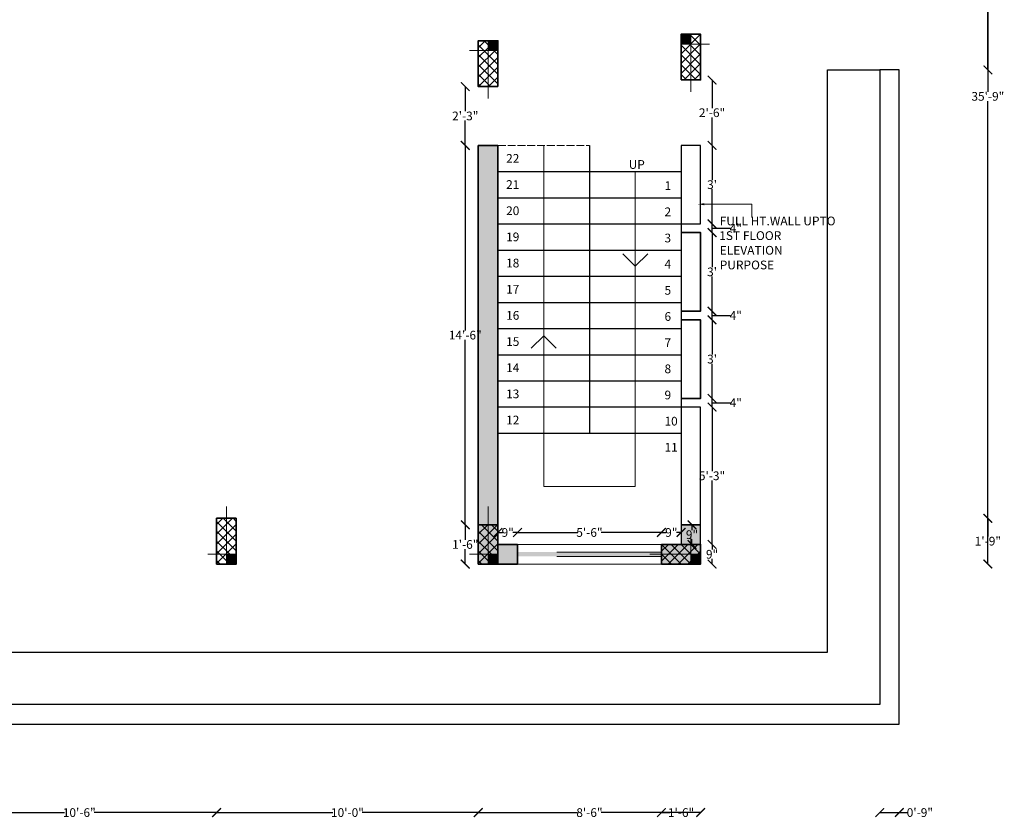
# Model space of a CAD drawing. Units: inches. Extents: x 2 to 905, y 9 to 678.
# Tile 7 of 8: x 454 to 905, y 12 to 378. Entities that reach past the tile are written whole.
import ezdxf

# ---------------------------------------------------------------- set-up
doc = ezdxf.new("R2010")
doc.units = ezdxf.units.IN
doc.linetypes.add('ACAD_ISO02W100', pattern=[15, 12, -3])
for name, color, linetype, lineweight in [('A-ANNO-DIMS', 7, 'Continuous', 18), ('A-ANNO-SYMB', 7, 'Continuous', 18), ('A-COLS', 1, 'Continuous', 35), ('A-COLS-MARK', 1, 'Continuous', 18), ('A-COLS-MARK-PATT', 3, 'Continuous', 13), ('A-COLS-PATT', 1, 'Continuous', 13), ('A-FLOR-STRS', 7, 'Continuous', 25), ('A-FLOR-STRS-HIDN', 7, 'ACAD_ISO02W100', 18), ('A-GLAZ', 4, 'Continuous', 18), ('A-GLAZ-PATT', 4, 'Continuous', 13), ('A-WALL', 7, 'Continuous', 35), ('C-PROP', 7, 'Continuous', 25)]:
    doc.layers.add(name, color=color, linetype=linetype, lineweight=lineweight)
doc.layers.add('A-ANNO-TEXT', color=251, linetype='Continuous', lineweight=18, true_color=0x636466)
doc.layers.add('A-WALL-PATT', color=252, linetype='Continuous', lineweight=13, true_color=0x939598)
doc.styles.add('PDF ArialMT', font='arial.ttf')
doc.styles.get("Standard").update_dxf_attribs({"font": 'arial.ttf'})
doc.dimstyles.get("Standard").update_dxf_attribs({"dimtxt": 4, "dimasz": 4, "dimexe": 0.18, "dimexo": 0.0625, "dimgap": 0.09, "dimtad": 0, "dimtih": 1, "dimtoh": 1, "dimdec": 1, "dimzin": 0, "dimdsep": 46, "dimlunit": 3, "dimtxsty": 'Standard', "dimblk": 'ARCHTICK', "dimcen": 0, "dimse1": 1, "dimse2": 1, "dimclrt": 1, "dimadec": 0, "dimazin": 0, "dimtfac": 1, "dimtdec": 1, "dimtofl": 0, "dimtmove": 0, "dimatfit": 3, "dimfxl": 1, "dimtolj": 1, "dimtzin": 0, "dimarcsym": 0})

# ---------------------------------------------------------------- blocks, each defined once
blk = doc.blocks.new('_ArchTick')
at = {"color": 0, "linetype": 'ByBlock', "const_width": 0.15}
blk.add_lwpolyline([(-0.5, -0.5), (0.5, 0.5)], dxfattribs=at)
blk = doc.blocks.new('*D67')
at = {"layer": 'A-ANNO-DIMS', "color": 0, "lineweight": -2, "transparency": 16777216}
for p, q in [((657.96, 146.58), (657.96, 139.71)), ((657.96, 128.58), (657.96, 135.45))]:
    blk.add_line(p, q, dxfattribs=at)
at = {"layer": 'Defpoints', "color": 0, "transparency": 16777216}
for p in [(657.96, 146.58), (663.93, 146.58), (663.93, 128.58)]:
    blk.add_point(p, dxfattribs=at)
at = {"layer": 'A-ANNO-DIMS', "color": 0, "lineweight": -2, "transparency": 16777216, "xscale": 4, "yscale": 4, "zscale": 4}
for p, rotation in [((657.96, 146.58), 90), ((657.96, 128.58), 270)]:
    blk.add_blockref('_ArchTick', p, dxfattribs=dict(at, rotation=rotation))
at = {"layer": 'A-ANNO-DIMS', "color": 0, "transparency": 16777216, "insert": (657.96, 137.58), "char_height": 4, "attachment_point": 5}
blk.add_mtext('\\A1;1\'-6"', dxfattribs=at)
blk = doc.blocks.new('*D68')
at = {"layer": 'A-ANNO-DIMS', "color": 0, "lineweight": -2, "transparency": 16777216}
for p, q in [((657.96, 320.58), (657.96, 235.71)), ((657.96, 146.58), (657.96, 231.45))]:
    blk.add_line(p, q, dxfattribs=at)
at = {"layer": 'Defpoints', "color": 0, "transparency": 16777216}
for p in [(657.96, 320.58), (663.93, 320.58), (663.93, 146.58)]:
    blk.add_point(p, dxfattribs=at)
at = {"layer": 'A-ANNO-DIMS', "color": 0, "lineweight": -2, "transparency": 16777216, "xscale": 4, "yscale": 4, "zscale": 4}
for p, rotation in [((657.96, 320.58), 90), ((657.96, 146.58), 270)]:
    blk.add_blockref('_ArchTick', p, dxfattribs=dict(at, rotation=rotation))
at = {"layer": 'A-ANNO-DIMS', "color": 0, "transparency": 16777216, "insert": (657.96, 233.58), "char_height": 4, "attachment_point": 5}
blk.add_mtext('\\A1;14\'-6"', dxfattribs=at)
blk = doc.blocks.new('*D69')
at = {"layer": 'A-ANNO-DIMS', "color": 0, "lineweight": -2, "transparency": 16777216}
for p, q in [((657.96, 347.58), (657.96, 336.21)), ((657.96, 320.58), (657.96, 331.94))]:
    blk.add_line(p, q, dxfattribs=at)
at = {"layer": 'Defpoints', "color": 0, "transparency": 16777216}
for p in [(657.96, 347.58), (663.93, 347.58), (663.93, 320.58)]:
    blk.add_point(p, dxfattribs=at)
at = {"layer": 'A-ANNO-DIMS', "color": 0, "lineweight": -2, "transparency": 16777216, "xscale": 4, "yscale": 4, "zscale": 4}
for p, rotation in [((657.96, 347.58), 90), ((657.96, 320.58), 270)]:
    blk.add_blockref('_ArchTick', p, dxfattribs=dict(at, rotation=rotation))
at = {"layer": 'A-ANNO-DIMS', "color": 0, "transparency": 16777216, "insert": (657.96, 334.08), "char_height": 4, "attachment_point": 5}
blk.add_mtext('\\A1;2\'-3"', dxfattribs=at)
blk = doc.blocks.new('*D70')
at = {"layer": 'A-ANNO-DIMS', "color": 0, "lineweight": -2, "transparency": 16777216}
for p, q in [((771.16, 137.58), (771.16, 135.21)), ((771.16, 128.58), (771.16, 130.95))]:
    blk.add_line(p, q, dxfattribs=at)
at = {"layer": 'Defpoints', "color": 0, "transparency": 16777216}
for p in [(765.93, 137.58), (771.16, 137.58), (765.93, 128.58)]:
    blk.add_point(p, dxfattribs=at)
at = {"layer": 'A-ANNO-DIMS', "color": 0, "lineweight": -2, "transparency": 16777216, "xscale": 4, "yscale": 4, "zscale": 4}
for p, rotation in [((771.16, 137.58), 90), ((771.16, 128.58), 270)]:
    blk.add_blockref('_ArchTick', p, dxfattribs=dict(at, rotation=rotation))
at = {"layer": 'A-ANNO-DIMS', "color": 0, "transparency": 16777216, "insert": (771.16, 133.08), "char_height": 4, "attachment_point": 5}
blk.add_mtext('\\A1;9"', dxfattribs=at)
blk = doc.blocks.new('*D71')
at = {"layer": 'A-ANNO-DIMS', "color": 0, "lineweight": -2, "transparency": 16777216}
for p, q in [((771.16, 200.58), (771.16, 171.21)), ((771.16, 137.58), (771.16, 166.94))]:
    blk.add_line(p, q, dxfattribs=at)
at = {"layer": 'Defpoints', "color": 0, "transparency": 16777216}
for p in [(765.93, 200.58), (771.16, 200.58), (765.93, 137.58)]:
    blk.add_point(p, dxfattribs=at)
at = {"layer": 'A-ANNO-DIMS', "color": 0, "lineweight": -2, "transparency": 16777216, "xscale": 4, "yscale": 4, "zscale": 4}
for p, rotation in [((771.16, 200.58), 90), ((771.16, 137.58), 270)]:
    blk.add_blockref('_ArchTick', p, dxfattribs=dict(at, rotation=rotation))
at = {"layer": 'A-ANNO-DIMS', "color": 0, "transparency": 16777216, "insert": (771.16, 169.08), "char_height": 4, "attachment_point": 5}
blk.add_mtext('\\A1;5\'-3"', dxfattribs=at)
blk = doc.blocks.new('*D72')
at = {"layer": 'A-ANNO-DIMS', "color": 0, "lineweight": -2, "transparency": 16777216}
for p, q in [((771.16, 200.58), (771.16, 204.58)), ((771.16, 202.58), (779.38, 202.58)), ((779.38, 202.58), (779.56, 202.58))]:
    blk.add_line(p, q, dxfattribs=at)
at = {"layer": 'Defpoints', "color": 0, "transparency": 16777216}
for p in [(765.93, 204.58), (771.16, 204.58), (765.93, 200.58)]:
    blk.add_point(p, dxfattribs=at)
at = {"layer": 'A-ANNO-DIMS', "color": 0, "lineweight": -2, "transparency": 16777216, "xscale": 4, "yscale": 4, "zscale": 4}
for p, rotation in [((771.16, 204.58), 90), ((771.16, 200.58), 270)]:
    blk.add_blockref('_ArchTick', p, dxfattribs=dict(at, rotation=rotation))
at = {"layer": 'A-ANNO-DIMS', "color": 0, "transparency": 16777216, "insert": (782.03, 202.58), "char_height": 4, "attachment_point": 5}
blk.add_mtext('\\A1;4"', dxfattribs=at)
blk = doc.blocks.new('*D73')
at = {"layer": 'A-ANNO-DIMS', "color": 0, "lineweight": -2, "transparency": 16777216}
for p, q in [((771.16, 240.58), (771.16, 224.71)), ((771.16, 204.58), (771.16, 220.44))]:
    blk.add_line(p, q, dxfattribs=at)
at = {"layer": 'Defpoints', "color": 0, "transparency": 16777216}
for p in [(765.93, 240.58), (771.16, 240.58), (765.93, 204.58)]:
    blk.add_point(p, dxfattribs=at)
at = {"layer": 'A-ANNO-DIMS', "color": 0, "lineweight": -2, "transparency": 16777216, "xscale": 4, "yscale": 4, "zscale": 4}
for p, rotation in [((771.16, 240.58), 90), ((771.16, 204.58), 270)]:
    blk.add_blockref('_ArchTick', p, dxfattribs=dict(at, rotation=rotation))
at = {"layer": 'A-ANNO-DIMS', "color": 0, "transparency": 16777216, "insert": (771.16, 222.58), "char_height": 4, "attachment_point": 5}
blk.add_mtext("\\A1;3'", dxfattribs=at)
blk = doc.blocks.new('*D74')
at = {"layer": 'A-ANNO-DIMS', "color": 0, "lineweight": -2, "transparency": 16777216}
for p, q in [((771.16, 240.58), (771.16, 244.58)), ((771.16, 242.58), (779.38, 242.58)), ((779.38, 242.58), (779.56, 242.58))]:
    blk.add_line(p, q, dxfattribs=at)
at = {"layer": 'Defpoints', "color": 0, "transparency": 16777216}
for p in [(765.93, 244.58), (771.16, 244.58), (765.93, 240.58)]:
    blk.add_point(p, dxfattribs=at)
at = {"layer": 'A-ANNO-DIMS', "color": 0, "lineweight": -2, "transparency": 16777216, "xscale": 4, "yscale": 4, "zscale": 4}
for p, rotation in [((771.16, 244.58), 90), ((771.16, 240.58), 270)]:
    blk.add_blockref('_ArchTick', p, dxfattribs=dict(at, rotation=rotation))
at = {"layer": 'A-ANNO-DIMS', "color": 0, "transparency": 16777216, "insert": (782.03, 242.58), "char_height": 4, "attachment_point": 5}
blk.add_mtext('\\A1;4"', dxfattribs=at)
blk = doc.blocks.new('*D75')
at = {"layer": 'A-ANNO-DIMS', "color": 0, "lineweight": -2, "transparency": 16777216}
for p, q in [((771.16, 280.58), (771.16, 264.71)), ((771.16, 244.58), (771.16, 260.44))]:
    blk.add_line(p, q, dxfattribs=at)
at = {"layer": 'Defpoints', "color": 0, "transparency": 16777216}
for p in [(765.93, 280.58), (771.16, 280.58), (765.93, 244.58)]:
    blk.add_point(p, dxfattribs=at)
at = {"layer": 'A-ANNO-DIMS', "color": 0, "lineweight": -2, "transparency": 16777216, "xscale": 4, "yscale": 4, "zscale": 4}
for p, rotation in [((771.16, 280.58), 90), ((771.16, 244.58), 270)]:
    blk.add_blockref('_ArchTick', p, dxfattribs=dict(at, rotation=rotation))
at = {"layer": 'A-ANNO-DIMS', "color": 0, "transparency": 16777216, "insert": (771.16, 262.58), "char_height": 4, "attachment_point": 5}
blk.add_mtext("\\A1;3'", dxfattribs=at)
blk = doc.blocks.new('*D76')
at = {"layer": 'A-ANNO-DIMS', "color": 0, "lineweight": -2, "transparency": 16777216}
for p, q in [((771.16, 280.58), (771.16, 284.58)), ((771.16, 282.58), (779.38, 282.58)), ((779.38, 282.58), (779.56, 282.58))]:
    blk.add_line(p, q, dxfattribs=at)
at = {"layer": 'Defpoints', "color": 0, "transparency": 16777216}
for p in [(765.93, 284.58), (771.16, 284.58), (765.93, 280.58)]:
    blk.add_point(p, dxfattribs=at)
at = {"layer": 'A-ANNO-DIMS', "color": 0, "lineweight": -2, "transparency": 16777216, "xscale": 4, "yscale": 4, "zscale": 4}
for p, rotation in [((771.16, 284.58), 90), ((771.16, 280.58), 270)]:
    blk.add_blockref('_ArchTick', p, dxfattribs=dict(at, rotation=rotation))
at = {"layer": 'A-ANNO-DIMS', "color": 0, "transparency": 16777216, "insert": (782.03, 282.58), "char_height": 4, "attachment_point": 5}
blk.add_mtext('\\A1;4"', dxfattribs=at)
blk = doc.blocks.new('*D77')
at = {"layer": 'A-ANNO-DIMS', "color": 0, "lineweight": -2, "transparency": 16777216}
for p, q in [((771.16, 320.58), (771.16, 304.71)), ((771.16, 284.58), (771.16, 300.44))]:
    blk.add_line(p, q, dxfattribs=at)
at = {"layer": 'Defpoints', "color": 0, "transparency": 16777216}
for p in [(765.93, 320.58), (771.16, 320.58), (765.93, 284.58)]:
    blk.add_point(p, dxfattribs=at)
at = {"layer": 'A-ANNO-DIMS', "color": 0, "lineweight": -2, "transparency": 16777216, "xscale": 4, "yscale": 4, "zscale": 4}
for p, rotation in [((771.16, 320.58), 90), ((771.16, 284.58), 270)]:
    blk.add_blockref('_ArchTick', p, dxfattribs=dict(at, rotation=rotation))
at = {"layer": 'A-ANNO-DIMS', "color": 0, "transparency": 16777216, "insert": (771.16, 302.58), "char_height": 4, "attachment_point": 5}
blk.add_mtext("\\A1;3'", dxfattribs=at)
blk = doc.blocks.new('*D78')
at = {"layer": 'A-ANNO-DIMS', "color": 0, "lineweight": -2, "transparency": 16777216}
for p, q in [((771.16, 350.58), (771.16, 337.71)), ((771.16, 320.58), (771.16, 333.45))]:
    blk.add_line(p, q, dxfattribs=at)
at = {"layer": 'Defpoints', "color": 0, "transparency": 16777216}
for p in [(765.93, 350.58), (771.16, 350.58), (765.93, 320.58)]:
    blk.add_point(p, dxfattribs=at)
at = {"layer": 'A-ANNO-DIMS', "color": 0, "lineweight": -2, "transparency": 16777216, "xscale": 4, "yscale": 4, "zscale": 4}
for p, rotation in [((771.16, 350.58), 90), ((771.16, 320.58), 270)]:
    blk.add_blockref('_ArchTick', p, dxfattribs=dict(at, rotation=rotation))
at = {"layer": 'A-ANNO-DIMS', "color": 0, "transparency": 16777216, "insert": (771.16, 335.58), "char_height": 4, "attachment_point": 5}
blk.add_mtext('\\A1;2\'-6"', dxfattribs=at)
blk = doc.blocks.new('*D79')
at = {"layer": 'A-ANNO-DIMS', "color": 0, "lineweight": -2, "transparency": 16777216}
for p, q in [((672.93, 143.07), (675.04, 143.07)), ((681.93, 143.07), (679.82, 143.07))]:
    blk.add_line(p, q, dxfattribs=at)
at = {"layer": 'Defpoints', "color": 0, "transparency": 16777216}
for p in [(681.93, 143.07), (672.93, 137.58), (681.93, 137.58)]:
    blk.add_point(p, dxfattribs=at)
at = {"layer": 'A-ANNO-DIMS', "color": 0, "lineweight": -2, "transparency": 16777216, "xscale": 4, "yscale": 4, "zscale": 4, "rotation": 180}
blk.add_blockref('_ArchTick', (672.93, 143.07), dxfattribs=at)
at = {"layer": 'A-ANNO-DIMS', "color": 0, "lineweight": -2, "transparency": 16777216, "xscale": 4, "yscale": 4, "zscale": 4}
blk.add_blockref('_ArchTick', (681.93, 143.07), dxfattribs=at)
at = {"layer": 'A-ANNO-DIMS', "color": 0, "transparency": 16777216, "insert": (677.43, 143.07), "char_height": 4, "attachment_point": 5}
blk.add_mtext('\\A1;9"', dxfattribs=at)
blk = doc.blocks.new('*D80')
at = {"layer": 'A-ANNO-DIMS', "color": 0, "lineweight": -2, "transparency": 16777216}
for p, q in [((747.98, 143.07), (750.08, 143.07)), ((756.96, 143.07), (754.86, 143.07))]:
    blk.add_line(p, q, dxfattribs=at)
at = {"layer": 'Defpoints', "color": 0, "transparency": 16777216}
for p in [(756.96, 143.07), (747.98, 137.58), (756.96, 137.58)]:
    blk.add_point(p, dxfattribs=at)
at = {"layer": 'A-ANNO-DIMS', "color": 0, "lineweight": -2, "transparency": 16777216, "xscale": 4, "yscale": 4, "zscale": 4, "rotation": 180}
blk.add_blockref('_ArchTick', (747.98, 143.07), dxfattribs=at)
at = {"layer": 'A-ANNO-DIMS', "color": 0, "lineweight": -2, "transparency": 16777216, "xscale": 4, "yscale": 4, "zscale": 4}
blk.add_blockref('_ArchTick', (756.96, 143.07), dxfattribs=at)
at = {"layer": 'A-ANNO-DIMS', "color": 0, "transparency": 16777216, "insert": (752.47, 143.07), "char_height": 4, "attachment_point": 5}
blk.add_mtext('\\A1;9"', dxfattribs=at)
blk = doc.blocks.new('*D81')
at = {"layer": 'A-ANNO-DIMS', "color": 0, "lineweight": -2, "transparency": 16777216}
for p, q in [((761.95, 146.58), (761.95, 144.21)), ((761.95, 137.58), (761.95, 139.95))]:
    blk.add_line(p, q, dxfattribs=at)
at = {"layer": 'Defpoints', "color": 0, "transparency": 16777216}
for p in [(756.93, 146.58), (761.95, 146.58), (756.93, 137.58)]:
    blk.add_point(p, dxfattribs=at)
at = {"layer": 'A-ANNO-DIMS', "color": 0, "lineweight": -2, "transparency": 16777216, "xscale": 4, "yscale": 4, "zscale": 4}
for p, rotation in [((761.95, 146.58), 90), ((761.95, 137.58), 270)]:
    blk.add_blockref('_ArchTick', p, dxfattribs=dict(at, rotation=rotation))
at = {"layer": 'A-ANNO-DIMS', "color": 0, "transparency": 16777216, "insert": (761.95, 142.08), "char_height": 4, "attachment_point": 5}
blk.add_mtext('\\A1;9"', dxfattribs=at)
blk = doc.blocks.new('*D82')
at = {"layer": 'A-ANNO-DIMS', "color": 0, "lineweight": -2, "transparency": 16777216}
for p, q in [((681.93, 143.07), (709.53, 143.07)), ((747.93, 143.07), (720.34, 143.07))]:
    blk.add_line(p, q, dxfattribs=at)
at = {"layer": 'Defpoints', "color": 0, "transparency": 16777216}
for p in [(747.93, 143.07), (681.93, 137.58), (747.93, 137.58)]:
    blk.add_point(p, dxfattribs=at)
at = {"layer": 'A-ANNO-DIMS', "color": 0, "lineweight": -2, "transparency": 16777216, "xscale": 4, "yscale": 4, "zscale": 4, "rotation": 180}
blk.add_blockref('_ArchTick', (681.93, 143.07), dxfattribs=at)
at = {"layer": 'A-ANNO-DIMS', "color": 0, "lineweight": -2, "transparency": 16777216, "xscale": 4, "yscale": 4, "zscale": 4}
blk.add_blockref('_ArchTick', (747.93, 143.07), dxfattribs=at)
at = {"layer": 'A-ANNO-DIMS', "color": 0, "transparency": 16777216, "insert": (714.93, 143.07), "char_height": 4, "attachment_point": 5}
blk.add_mtext('\\A1;5\'-6"', dxfattribs=at)
blk = doc.blocks.new('COL-DATUM-R')
h = blk.add_hatch(color=256)
h.dxf.hatch_style = 1
h.paths.add_polyline_path([(13.01, 0), (13.01, 4.5), (8.51, 4.5), (8.51, 0)])
for p, q in [((8.51, 0), (8.51, 26.48)), ((13.01, 4.5), (0, 4.5))]:
    blk.add_line(p, q)
blk.add_lwpolyline([(8.51, 0), (13.01, 0), (13.01, 4.5), (8.51, 4.5)], close=True)
blk = doc.blocks.new('COL-DATUM-L')
h = blk.add_hatch(color=256)
h.dxf.hatch_style = 1
h.paths.add_polyline_path([(4.5, 0), (4.5, 4.5), (0, 4.5), (0, 0)])
for p, q in [((4.5, 0), (4.5, 26.48)), ((0, 4.5), (13.01, 4.5))]:
    blk.add_line(p, q)
blk.add_lwpolyline([(4.5, 0), (0, 0), (0, 4.5), (4.5, 4.5)], close=True)
blk = doc.blocks.new('COL-DATUM-CROSS-SHORT')
for p, q in [((18.83, 0), (18.83, 13.01)), ((23.33, 4.5), (0, 4.5))]:
    blk.add_line(p, q)
blk = doc.blocks.new('*D104')
at = {"layer": 'A-ANNO-DIMS', "color": 0, "lineweight": -2, "transparency": 16777216}
for p, q in [((897.65, 535.22), (897.65, 447.35)), ((897.65, 355.22), (897.65, 443.09))]:
    blk.add_line(p, q, dxfattribs=at)
at = {"layer": 'Defpoints', "color": 0, "transparency": 16777216}
for p in [(857.05, 535.22), (897.65, 535.22), (857.05, 355.22)]:
    blk.add_point(p, dxfattribs=at)
at = {"layer": 'A-ANNO-DIMS', "color": 0, "lineweight": -2, "transparency": 16777216, "xscale": 4, "yscale": 4, "zscale": 4}
for p, rotation in [((897.65, 535.22), 90), ((897.65, 355.22), 270)]:
    blk.add_blockref('_ArchTick', p, dxfattribs=dict(at, rotation=rotation))
at = {"layer": 'A-ANNO-DIMS', "color": 1, "transparency": 16777216, "insert": (897.65, 445.22), "char_height": 4, "attachment_point": 5}
blk.add_mtext('\\A1;15\'-0"', dxfattribs=at)
blk = doc.blocks.new('*D106')
at = {"layer": 'A-ANNO-DIMS', "color": 0, "lineweight": -2, "transparency": 16777216}
for p, q in [((848.05, 14.62), (857.05, 14.62)), ((857.05, 14.62), (861.05, 14.62))]:
    blk.add_line(p, q, dxfattribs=at)
at = {"layer": 'Defpoints', "color": 0, "transparency": 16777216}
for p in [(848.05, 535.22), (857.05, 535.22), (857.05, 14.62)]:
    blk.add_point(p, dxfattribs=at)
at = {"layer": 'A-ANNO-DIMS', "color": 0, "lineweight": -2, "transparency": 16777216, "xscale": 4, "yscale": 4, "zscale": 4, "rotation": 180}
blk.add_blockref('_ArchTick', (848.05, 14.62), dxfattribs=at)
at = {"layer": 'A-ANNO-DIMS', "color": 0, "lineweight": -2, "transparency": 16777216, "xscale": 4, "yscale": 4, "zscale": 4}
blk.add_blockref('_ArchTick', (857.05, 14.62), dxfattribs=at)
at = {"layer": 'A-ANNO-DIMS', "color": 1, "transparency": 16777216, "insert": (866.46, 14.62), "char_height": 4, "attachment_point": 5}
blk.add_mtext('\\A1;0\'-9"', dxfattribs=at)
blk = doc.blocks.new('*D112')
at = {"layer": 'A-ANNO-DIMS', "color": 0, "lineweight": -2, "transparency": 16777216}
for p, q in [((897.65, 557.58), (897.65, 345.21)), ((897.65, 128.58), (897.65, 340.94))]:
    blk.add_line(p, q, dxfattribs=at)
at = {"layer": 'Defpoints', "color": 0, "transparency": 16777216}
for p in [(417.93, 557.58), (897.65, 557.58), (417.93, 128.58)]:
    blk.add_point(p, dxfattribs=at)
at = {"layer": 'A-ANNO-DIMS', "color": 0, "lineweight": -2, "transparency": 16777216, "xscale": 4, "yscale": 4, "zscale": 4}
for p, rotation in [((897.65, 557.58), 90), ((897.65, 128.58), 270)]:
    blk.add_blockref('_ArchTick', p, dxfattribs=dict(at, rotation=rotation))
at = {"layer": 'A-ANNO-DIMS', "color": 1, "transparency": 16777216, "insert": (897.65, 343.08), "char_height": 4, "attachment_point": 5}
blk.add_mtext('\\A1;35\'-9"', dxfattribs=at)
blk = doc.blocks.new('*D114')
at = {"layer": 'A-ANNO-DIMS', "color": 0, "lineweight": -2, "transparency": 16777216}
for p, q in [((417.93, 14.62), (474.16, 14.62)), ((543.93, 14.62), (487.71, 14.62))]:
    blk.add_line(p, q, dxfattribs=at)
at = {"layer": 'Defpoints', "color": 0, "transparency": 16777216}
for p in [(417.93, 128.58), (543.93, 128.58), (543.93, 14.62)]:
    blk.add_point(p, dxfattribs=at)
at = {"layer": 'A-ANNO-DIMS', "color": 0, "lineweight": -2, "transparency": 16777216, "xscale": 4, "yscale": 4, "zscale": 4, "rotation": 180}
blk.add_blockref('_ArchTick', (417.93, 14.62), dxfattribs=at)
at = {"layer": 'A-ANNO-DIMS', "color": 0, "lineweight": -2, "transparency": 16777216, "xscale": 4, "yscale": 4, "zscale": 4}
blk.add_blockref('_ArchTick', (543.93, 14.62), dxfattribs=at)
at = {"layer": 'A-ANNO-DIMS', "color": 1, "transparency": 16777216, "insert": (480.93, 14.62), "char_height": 4, "attachment_point": 5}
blk.add_mtext('\\A1;10\'-6"', dxfattribs=at)
blk = doc.blocks.new('*D115')
at = {"layer": 'A-ANNO-DIMS', "color": 0, "lineweight": -2, "transparency": 16777216}
for p, q in [((543.93, 14.62), (597.16, 14.62)), ((663.93, 14.62), (610.71, 14.62))]:
    blk.add_line(p, q, dxfattribs=at)
at = {"layer": 'Defpoints', "color": 0, "transparency": 16777216}
for p in [(543.93, 128.58), (663.93, 128.58), (663.93, 14.62)]:
    blk.add_point(p, dxfattribs=at)
at = {"layer": 'A-ANNO-DIMS', "color": 0, "lineweight": -2, "transparency": 16777216, "xscale": 4, "yscale": 4, "zscale": 4, "rotation": 180}
blk.add_blockref('_ArchTick', (543.93, 14.62), dxfattribs=at)
at = {"layer": 'A-ANNO-DIMS', "color": 0, "lineweight": -2, "transparency": 16777216, "xscale": 4, "yscale": 4, "zscale": 4}
blk.add_blockref('_ArchTick', (663.93, 14.62), dxfattribs=at)
at = {"layer": 'A-ANNO-DIMS', "color": 1, "transparency": 16777216, "insert": (603.93, 14.62), "char_height": 4, "attachment_point": 5}
blk.add_mtext('\\A1;10\'-0"', dxfattribs=at)
blk = doc.blocks.new('*D116')
at = {"layer": 'A-ANNO-DIMS', "color": 0, "lineweight": -2, "transparency": 16777216}
for p, q in [((663.93, 14.62), (709.52, 14.62)), ((765.93, 14.62), (720.34, 14.62))]:
    blk.add_line(p, q, dxfattribs=at)
at = {"layer": 'Defpoints', "color": 0, "transparency": 16777216}
for p in [(663.93, 128.58), (765.93, 128.58), (765.93, 14.62)]:
    blk.add_point(p, dxfattribs=at)
at = {"layer": 'A-ANNO-DIMS', "color": 0, "lineweight": -2, "transparency": 16777216, "xscale": 4, "yscale": 4, "zscale": 4, "rotation": 180}
blk.add_blockref('_ArchTick', (663.93, 14.62), dxfattribs=at)
at = {"layer": 'A-ANNO-DIMS', "color": 0, "lineweight": -2, "transparency": 16777216, "xscale": 4, "yscale": 4, "zscale": 4}
blk.add_blockref('_ArchTick', (765.93, 14.62), dxfattribs=at)
at = {"layer": 'A-ANNO-DIMS', "color": 1, "transparency": 16777216, "insert": (714.93, 14.62), "char_height": 4, "attachment_point": 5}
blk.add_mtext('\\A1;8\'-6"', dxfattribs=at)
blk = doc.blocks.new('*D117')
at = {"layer": 'A-ANNO-DIMS', "color": 0, "lineweight": -2, "transparency": 16777216}
for p, q in [((543.93, 671.82), (552.93, 671.82)), ((552.93, 671.82), (556.93, 671.82))]:
    blk.add_line(p, q, dxfattribs=at)
at = {"layer": 'Defpoints', "color": 0, "transparency": 16777216}
for p in [(552.93, 671.82), (543.93, 149.58), (552.93, 149.58)]:
    blk.add_point(p, dxfattribs=at)
at = {"layer": 'A-ANNO-DIMS', "color": 0, "lineweight": -2, "transparency": 16777216, "xscale": 4, "yscale": 4, "zscale": 4, "rotation": 180}
blk.add_blockref('_ArchTick', (543.93, 671.82), dxfattribs=at)
at = {"layer": 'A-ANNO-DIMS', "color": 0, "lineweight": -2, "transparency": 16777216, "xscale": 4, "yscale": 4, "zscale": 4}
blk.add_blockref('_ArchTick', (552.93, 671.82), dxfattribs=at)
at = {"layer": 'A-ANNO-DIMS', "color": 1, "transparency": 16777216, "insert": (562.34, 671.82), "char_height": 4, "attachment_point": 5}
blk.add_mtext('\\A1;0\'-9"', dxfattribs=at)
blk = doc.blocks.new('*D118')
at = {"layer": 'A-ANNO-DIMS', "color": 0, "lineweight": -2, "transparency": 16777216}
for p, q in [((897.65, 149.58), (897.65, 141.21)), ((897.65, 128.58), (897.65, 136.95))]:
    blk.add_line(p, q, dxfattribs=at)
at = {"layer": 'Defpoints', "color": 0, "transparency": 16777216}
for p in [(552.93, 149.58), (897.65, 149.58), (552.93, 128.58)]:
    blk.add_point(p, dxfattribs=at)
at = {"layer": 'A-ANNO-DIMS', "color": 0, "lineweight": -2, "transparency": 16777216, "xscale": 4, "yscale": 4, "zscale": 4}
for p, rotation in [((897.65, 149.58), 90), ((897.65, 128.58), 270)]:
    blk.add_blockref('_ArchTick', p, dxfattribs=dict(at, rotation=rotation))
at = {"layer": 'A-ANNO-DIMS', "color": 1, "transparency": 16777216, "insert": (897.65, 139.08), "char_height": 4, "attachment_point": 5}
blk.add_mtext('\\A1;1\'-9"', dxfattribs=at)
blk = doc.blocks.new('*D119')
at = {"layer": 'A-ANNO-DIMS', "color": 0, "lineweight": -2, "transparency": 16777216}
for p, q in [((747.93, 14.62), (751.72, 14.62)), ((765.93, 14.62), (762.15, 14.62))]:
    blk.add_line(p, q, dxfattribs=at)
at = {"layer": 'Defpoints', "color": 0, "transparency": 16777216}
for p in [(747.93, 548.58), (765.93, 548.58), (765.93, 14.62)]:
    blk.add_point(p, dxfattribs=at)
at = {"layer": 'A-ANNO-DIMS', "color": 0, "lineweight": -2, "transparency": 16777216, "xscale": 4, "yscale": 4, "zscale": 4, "rotation": 180}
blk.add_blockref('_ArchTick', (747.93, 14.62), dxfattribs=at)
at = {"layer": 'A-ANNO-DIMS', "color": 0, "lineweight": -2, "transparency": 16777216, "xscale": 4, "yscale": 4, "zscale": 4}
blk.add_blockref('_ArchTick', (765.93, 14.62), dxfattribs=at)
at = {"layer": 'A-ANNO-DIMS', "color": 1, "transparency": 16777216, "insert": (756.93, 14.62), "char_height": 4, "attachment_point": 5}
blk.add_mtext('\\A1;1\'-6"', dxfattribs=at)

msp = doc.modelspace()

# ---------------------------------------------------------------- hatches: boundary and pattern name
at = {"layer": 'A-COLS-MARK-PATT'}
h = msp.add_hatch(color=256, dxfattribs=at)
h.dxf.hatch_style = 1
h.paths.add_polyline_path([(765.93, 133.08), (761.43, 133.08), (761.43, 128.58), (765.93, 128.58)])
at = {"layer": 'A-COLS-PATT'}
h = msp.add_hatch(dxfattribs=at)
h.set_pattern_fill('ANSI37', color=256)
h.set_pattern_definition([(45, (1232.609, 3.1098), (-2.245064, 2.245064), []), (135, (1232.609, 3.1098), (-2.245064, -2.245064), [])])
h.paths.add_polyline_path([(765.93, 367.08), (761.43, 367.08), (761.43, 371.58), (765.93, 371.58)])
h.paths.add_polyline_path([(765.93, 350.58), (761.43, 350.58), (761.43, 367.08), (765.93, 367.08)])
h.paths.add_polyline_path([(761.43, 350.58), (756.93, 350.58), (756.93, 367.08), (761.43, 367.08)])
h = msp.add_hatch(dxfattribs=at)
h.set_pattern_fill('ANSI37', color=256)
h.set_pattern_definition([(45, (1232.609, 0.1098), (-2.245064, 2.245064), []), (135, (1232.609, 0.1098), (-2.245064, -2.245064), [])])
h.paths.add_polyline_path([(663.93, 364.08), (668.43, 364.08), (668.43, 368.58), (663.93, 368.58)])
h.paths.add_polyline_path([(663.93, 347.58), (668.43, 347.58), (668.43, 364.08), (663.93, 364.08)])
h.paths.add_polyline_path([(668.43, 347.58), (672.93, 347.58), (672.93, 364.08), (668.43, 364.08)])
h = msp.add_hatch(dxfattribs=at)
h.set_pattern_fill('ANSI37', color=256)
h.set_pattern_definition([(45, (1112.609, -47.8902), (-2.245064, 2.245064), []), (135, (1112.609, -47.8902), (-2.245064, -2.245064), [])])
h.paths.add_polyline_path([(543.93, 133.08), (548.43, 133.08), (548.43, 128.58), (543.93, 128.58)])
h.paths.add_polyline_path([(543.93, 149.58), (548.43, 149.58), (548.43, 133.08), (543.93, 133.08)])
h.paths.add_polyline_path([(548.43, 149.58), (552.93, 149.58), (552.93, 133.08), (548.43, 133.08)])
h = msp.add_hatch(dxfattribs=at)
h.set_pattern_fill('ANSI37', color=256)
h.set_pattern_definition([(45, (1232.609, -47.8902), (-2.245064, 2.245064), []), (135, (1232.609, -47.8902), (-2.245064, -2.245064), [])])
h.paths.add_polyline_path([(663.93, 133.08), (668.43, 133.08), (668.43, 128.58), (663.93, 128.58)])
h.paths.add_polyline_path([(672.93, 146.58), (668.43, 146.58), (668.43, 133.08), (672.93, 133.08)])
h.paths.add_polyline_path([(668.43, 146.58), (663.93, 146.58), (663.93, 133.08), (668.43, 133.08)])
h = msp.add_hatch(dxfattribs=at)
h.set_pattern_fill('ANSI37', color=256, angle=90)
h.set_pattern_definition([(135, (1041.4012, 706.2528), (-2.245064, -2.245064), []), (225, (1041.4012, 706.2528), (2.245064, -2.245064), [])])
h.paths.add_polyline_path([(761.43, 137.58), (761.43, 133.08), (765.93, 133.08), (765.93, 137.58)])
h.paths.add_polyline_path([(747.98, 128.58), (747.98, 133.08), (761.43, 133.08), (761.43, 128.58)])
h.paths.add_polyline_path([(747.98, 133.08), (747.98, 137.58), (761.43, 137.58), (761.43, 133.08)])
at = {"layer": 'A-GLAZ-PATT'}
h = msp.add_hatch(color=256, dxfattribs=at)
h.dxf.hatch_style = 1
h.paths.add_polyline_path([(747.93, 132.08), (747.93, 134.08), (681.93, 134.08), (681.93, 132.08)])
at = {"layer": 'A-WALL-PATT'}
h = msp.add_hatch(color=256, dxfattribs=at)
h.dxf.hatch_style = 1
h.paths.add_polyline_path([(672.93, 320.58), (663.93, 320.58), (663.93, 128.58), (681.93, 128.58), (681.93, 137.58), (672.93, 137.58)])
h = msp.add_hatch(color=256, dxfattribs=at)
h.dxf.hatch_style = 1
h.paths.add_polyline_path([(765.93, 146.58), (756.93, 146.58), (756.93, 137.58), (747.93, 137.58), (747.93, 128.58), (765.93, 128.58)])

# ---------------------------------------------------------------- linework, layer by layer
at = {"layer": 'A-ANNO-SYMB'}
for points in [[(735.93, 308.58), (735.93, 164.2), (693.93, 164.2), (693.93, 320.58)], [(741.63, 270.88), (735.93, 265.23), (730.23, 270.88)], [(699.63, 227.54), (693.93, 233.19), (688.23, 227.54)]]:
    msp.add_lwpolyline(points, dxfattribs=at)
at = {"layer": 'A-ANNO-TEXT'}
msp.add_lwpolyline([(767.69, 293.65), (789.41, 293.65), (789.41, 287.48)], dxfattribs=at)
at = {"layer": 'A-ANNO-TEXT', "transparency": 33554559}
msp.add_solid([(767.69, 293.1), (764.71, 293.65), (767.69, 294.09)], dxfattribs=at)
at = {"layer": 'A-COLS'}
for p, q in [((765.93, 371.58), (756.93, 371.58)), ((663.93, 368.58), (672.93, 368.58))]:
    msp.add_line(p, q, dxfattribs=at)
for points in [[(756.93, 350.58), (765.93, 350.58), (765.93, 371.58), (756.93, 371.58)], [(672.93, 347.58), (663.93, 347.58), (663.93, 368.58), (672.93, 368.58)], [(552.93, 149.58), (543.93, 149.58), (543.93, 128.58), (552.93, 128.58)], [(672.93, 146.58), (663.93, 146.58), (663.93, 128.58), (672.93, 128.58)], [(747.98, 128.58), (747.98, 137.58), (765.93, 137.58), (765.93, 128.58)]]:
    msp.add_lwpolyline(points, close=True, dxfattribs=at)
at = {"layer": 'A-COLS-MARK'}
msp.add_lwpolyline([(765.93, 133.08), (765.93, 128.58), (761.43, 128.58), (761.43, 133.08)], close=True, dxfattribs=at)
at = {"layer": 'A-FLOR-STRS'}
for p, q in [((714.93, 320.58), (714.93, 188.58)), ((672.93, 188.58), (714.93, 188.58)), ((714.93, 188.58), (756.93, 188.58))]:
    msp.add_line(p, q, dxfattribs=at)
for points in [[(672.93, 284.58), (714.93, 284.58), (756.93, 284.58), (765.93, 284.58), (765.93, 320.58), (756.93, 320.58), (756.93, 137.58)], [(672.93, 308.58), (714.93, 308.58), (756.93, 308.58)], [(672.93, 296.58), (714.93, 296.58), (756.93, 296.58)], [(672.93, 272.58), (714.93, 272.58), (756.93, 272.58)], [(672.93, 260.58), (714.93, 260.58), (756.93, 260.58)], [(672.93, 248.58), (714.93, 248.58), (756.93, 248.58)], [(672.93, 236.58), (714.93, 236.58), (756.93, 236.58)], [(672.93, 224.58), (714.93, 224.58), (756.93, 224.58)], [(672.93, 212.58), (714.93, 212.58), (756.93, 212.58)], [(747.93, 137.58), (756.93, 137.58), (765.93, 137.58), (765.93, 128.58), (765.93, 200.58), (756.93, 200.58), (714.93, 200.58), (672.93, 200.58)]]:
    msp.add_lwpolyline(points, dxfattribs=at)
at = {"layer": 'A-FLOR-STRS-HIDN', "ltscale": 0.3}
msp.add_line((672.93, 320.58), (714.93, 320.58), dxfattribs=at)
at = {"layer": 'A-GLAZ'}
for p, q in [((699.93, 134.08), (747.93, 134.08)), ((699.93, 132.08), (747.93, 132.08))]:
    msp.add_line(p, q, dxfattribs=at)
msp.add_lwpolyline([(681.93, 137.58), (747.93, 137.58), (747.93, 128.58), (681.93, 128.58)], close=True, dxfattribs=at)
at = {"layer": 'A-WALL'}
for p, q in [((663.93, 128.58), (663.93, 320.58)), ((672.93, 320.58), (663.93, 320.58)), ((672.93, 137.58), (672.93, 320.58)), ((756.93, 146.58), (765.93, 146.58)), ((672.93, 137.58), (681.93, 137.58)), ((681.93, 137.58), (681.93, 128.58)), ((663.93, 128.58), (681.93, 128.58)), ((747.93, 128.58), (765.93, 128.58))]:
    msp.add_line(p, q, dxfattribs=at)
for points in [[(756.93, 280.58), (765.93, 280.58), (765.93, 244.58), (756.93, 244.58)], [(756.93, 240.58), (765.93, 240.58), (765.93, 204.58), (756.93, 204.58)]]:
    msp.add_lwpolyline(points, dxfattribs=at)
msp.add_lwpolyline([(747.93, 137.58), (747.93, 128.58)], close=True, dxfattribs=at)
at = {"layer": 'C-PROP'}
msp.add_lwpolyline([(857.05, 535.22), (857.05, 631.22), (53.05, 631.22), (53.05, 55.22), (857.05, 55.22), (857.05, 355.22), (848.05, 355.22), (848.05, 64.22), (62.05, 64.22), (62.05, 622.22), (848.05, 622.22), (848.05, 535.22)], close=True, dxfattribs=at)
msp.add_lwpolyline([(848.05, 598.22), (86.05, 598.22), (86.05, 88.22), (824.05, 88.22), (824.05, 355.22), (836.05, 355.22), (848.05, 355.22)], dxfattribs=at)

# ---------------------------------------------------------------- block references
at = {"layer": 'A-COLS-MARK', "rotation": 180}
for name, p in [('COL-DATUM-R', (769.94, 371.58)), ('COL-DATUM-L', (672.93, 368.58))]:
    msp.add_blockref(name, p, dxfattribs=at)
at = {"layer": 'A-COLS-MARK'}
for name, p in [('COL-DATUM-R', (539.92, 128.58)), ('COL-DATUM-R', (659.92, 128.58)), ('COL-DATUM-CROSS-SHORT', (742.6, 128.58))]:
    msp.add_blockref(name, p, dxfattribs=at)

# ---------------------------------------------------------------- texts
at = {"layer": 'A-ANNO-SYMB', "char_height": 4, "attachment_point": 1}
for s, width, insert in [('22', 5.3905, (676.71, 316.63)), ('{\\fArial|b1|i0|c0|p34;UP}', 10.6286, (732.93, 313.83)), ('21', 5.3905, (676.71, 304.63)), ('1', 5.3905, (749.35, 304.12)), ('20', 5.3905, (676.71, 292.63)), ('2', 5.3905, (749.35, 292.12)), ('19', 5.3905, (676.71, 280.63)), ('3', 5.3905, (749.35, 280.12)), ('18', 5.3905, (676.71, 268.63)), ('4', 5.3905, (749.35, 268.12)), ('17', 5.3905, (676.71, 256.63)), ('5', 5.3905, (749.35, 256.12)), ('16', 5.3905, (676.71, 244.63)), ('6', 5.3905, (749.35, 244.12)), ('15', 5.3905, (676.71, 232.63)), ('7', 5.3905, (749.35, 232.12)), ('14', 5.3905, (676.71, 220.63)), ('8', 5.3905, (749.35, 220.12)), ('13', 5.3905, (676.71, 208.63)), ('9', 5.3905, (749.35, 208.12)), ('12', 5.3905, (676.71, 196.63)), ('10', 5.3905, (749.35, 196.12)), ('11', 5.3905, (749.35, 184.12))]:
    msp.add_mtext_dynamic_manual_height_columns(s, width=width, gutter_width=12.5, heights=[0], dxfattribs=dict(at, insert=insert))
at = {"layer": 'A-ANNO-TEXT', "attachment_point": 4, "style": 'PDF ArialMT'}
for s, insert, char_height in [('FULL HT.WALL UPTO', (774.67, 285.41), 4.0234), ('1ST FLOOR', (774.45, 278.69), 4.023), ('ELEVATION', (774.67, 271.96), 4.023), ('PURPOSE', (774.67, 265.23), 4.023)]:
    msp.add_mtext(s, dxfattribs=dict(at, insert=insert, char_height=char_height))

# ---------------------------------------------------------------- dimensions: what is measured, and where the dimension line sits
at = {"layer": 'A-ANNO-DIMS'}
for base, p1, p2, override, picture, middle in [((552.93, 671.82), (543.93, 149.58), (552.93, 149.58), {"dimdec": 1, "dimlfac": 1, "dimrnd": 0, "dimzin": 1, "dimdsep": 46, "dimlunit": 4, "dimfrac": 2}, '*D117', (562.34, 671.82)), ((765.93, 14.62), (747.93, 548.58), (765.93, 548.58), {"dimdec": 1, "dimlfac": 1, "dimrnd": 0, "dimzin": 1, "dimdsep": 46, "dimlunit": 4, "dimfrac": 2}, '*D119', (756.93, 14.62)), ((857.05, 14.62), (848.05, 535.22), (857.05, 535.22), {"dimdec": 1, "dimlfac": 1, "dimrnd": 0, "dimzin": 1, "dimdsep": 46, "dimlunit": 4, "dimfrac": 2}, '*D106', (866.46, 14.62)), ((681.93, 143.07), (672.93, 137.58), (681.93, 137.58), {"dimdec": 0, "dimclrd": 0, "dimclre": 0, "dimclrt": 0}, '*D79', (677.43, 143.07)), ((747.93, 143.07), (681.93, 137.58), (747.93, 137.58), {"dimdec": 0, "dimclrd": 0, "dimclre": 0, "dimclrt": 0}, '*D82', (714.93, 143.07)), ((756.96, 143.07), (747.98, 137.58), (756.96, 137.58), {"dimdec": 0, "dimclrd": 0, "dimclre": 0, "dimclrt": 0, "dimtmove": 1}, '*D80', (752.47, 143.07)), ((543.93, 14.62), (417.93, 128.58), (543.93, 128.58), {"dimdec": 1, "dimlfac": 1, "dimrnd": 0, "dimzin": 1, "dimdsep": 46, "dimlunit": 4, "dimfrac": 2}, '*D114', (480.93, 14.62)), ((663.93, 14.62), (543.93, 128.58), (663.93, 128.58), {"dimdec": 1, "dimlfac": 1, "dimrnd": 0, "dimzin": 1, "dimdsep": 46, "dimlunit": 4, "dimfrac": 2}, '*D115', (603.93, 14.62)), ((765.93, 14.62), (663.93, 128.58), (765.93, 128.58), {"dimdec": 1, "dimlfac": 1, "dimrnd": 0, "dimzin": 1, "dimdsep": 46, "dimlunit": 4, "dimfrac": 2}, '*D116', (714.93, 14.62))]:
    dim = msp.add_linear_dim(base=base, p1=p1, p2=p2, dimstyle='Standard', override=override, dxfattribs=at)
    dim.commit()
    dim.dimension.update_dxf_attribs({"geometry": picture, "text_midpoint": middle})
for base, p1, p2, override, picture, middle in [((897.65, 557.58), (417.93, 128.58), (417.93, 557.58), {"dimdec": 1, "dimlfac": 1, "dimrnd": 0, "dimzin": 1, "dimdsep": 46, "dimlunit": 4, "dimfrac": 2}, '*D112', (897.65, 343.08)), ((897.65, 535.22), (857.05, 355.22), (857.05, 535.22), {"dimdec": 1, "dimlfac": 1, "dimrnd": 0, "dimzin": 1, "dimdsep": 46, "dimlunit": 4, "dimfrac": 2}, '*D104', (897.65, 445.22)), ((771.16, 350.58), (765.93, 320.58), (765.93, 350.58), {"dimdec": 0, "dimclrd": 0, "dimclre": 0, "dimclrt": 0, "dimtmove": 1}, '*D78', (771.16, 335.58)), ((657.96, 347.58), (663.93, 320.58), (663.93, 347.58), {"dimdec": 0, "dimclrd": 0, "dimclre": 0, "dimclrt": 0, "dimtmove": 1}, '*D69', (657.96, 334.08)), ((657.96, 320.58), (663.93, 146.58), (663.93, 320.58), {"dimdec": 0, "dimclrd": 0, "dimclre": 0, "dimclrt": 0, "dimtmove": 1}, '*D68', (657.96, 233.58)), ((771.16, 320.58), (765.93, 284.58), (765.93, 320.58), {"dimclrd": 0, "dimclre": 0, "dimclrt": 0, "dimtmove": 1}, '*D77', (771.16, 302.58)), ((771.16, 284.58), (765.93, 280.58), (765.93, 284.58), {"dimdec": 0, "dimclrd": 0, "dimclre": 0, "dimclrt": 0, "dimtmove": 1}, '*D76', (779.65, 282.58)), ((771.16, 280.58), (765.93, 244.58), (765.93, 280.58), {"dimclrd": 0, "dimclre": 0, "dimclrt": 0, "dimtmove": 1}, '*D75', (771.16, 262.58)), ((771.16, 244.58), (765.93, 240.58), (765.93, 244.58), {"dimdec": 0, "dimclrd": 0, "dimclre": 0, "dimclrt": 0, "dimtmove": 1}, '*D74', (779.65, 242.58)), ((771.16, 240.58), (765.93, 204.58), (765.93, 240.58), {"dimclrd": 0, "dimclre": 0, "dimclrt": 0, "dimtmove": 1}, '*D73', (771.16, 222.58)), ((771.16, 204.58), (765.93, 200.58), (765.93, 204.58), {"dimdec": 0, "dimclrd": 0, "dimclre": 0, "dimclrt": 0, "dimtmove": 1}, '*D72', (779.65, 202.58)), ((771.16, 200.58), (765.93, 137.58), (765.93, 200.58), {"dimdec": 0, "dimclrd": 0, "dimclre": 0, "dimclrt": 0, "dimtmove": 1}, '*D71', (771.16, 169.08)), ((897.65, 149.58), (552.93, 128.58), (552.93, 149.58), {"dimdec": 1, "dimlfac": 1, "dimrnd": 0, "dimzin": 1, "dimdsep": 46, "dimlunit": 4, "dimfrac": 2}, '*D118', (897.65, 139.08)), ((657.96, 146.58), (663.93, 128.58), (663.93, 146.58), {"dimdec": 0, "dimclrd": 0, "dimclre": 0, "dimclrt": 0}, '*D67', (657.96, 137.58)), ((771.16, 137.58), (765.93, 128.58), (765.93, 137.58), {"dimdec": 0, "dimclrd": 0, "dimclre": 0, "dimclrt": 0}, '*D70', (771.16, 133.08))]:
    dim = msp.add_linear_dim(base=base, p1=p1, p2=p2, angle=90, dimstyle='Standard', override=override, dxfattribs=at)
    dim.commit()
    dim.dimension.update_dxf_attribs({"geometry": picture, "text_midpoint": middle})
dim = msp.add_linear_dim(base=(761.95, 146.58), p1=(756.93, 137.58), p2=(756.93, 146.58), angle=90, dimstyle='Standard', override={"dimdec": 0, "dimclrd": 0, "dimclre": 0, "dimclrt": 0}, dxfattribs=at)
dim.commit()
dim.dimension.update_dxf_attribs({"geometry": '*D81', "text_midpoint": (761.95, 142.08), "dimtype": 160})

doc.saveas('drawing.dxf')
